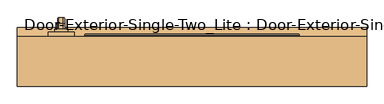
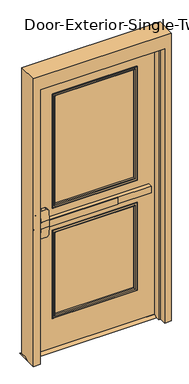
"""IFC4 building model written with IfcOpenShell, lengths in millimetres: door geometry, Door-Exterior-Single-Two_Lite : Door-Exterior-Single-Two_Lite."""

from ifc_helpers import new_model, si_unit, point, frame, frame_2d, origin, place, context, project, spatial, polyline, circle_curve, ellipse_curve, trimmed, segment, composite_curve, outline, extrude, faceted_brep, source, transform, mapped, element, save
from ifc_brep_helpers import plane_surface, cylinder_surface, revolved_surface, advanced_brep


def door_exterior_single_two_lite_door_exterior_single_two_lite_36a17ea7(model_context):
    return source(origin(), model_context, "Body", "SolidModel", [
        extrude(outline(polyline([(38.1, 12.7), (82.55, 12.7), (107.95, 0.0), (12.7, 0.0), (38.1, 12.7)])), frame((-508.0, 0.0, 0.0), z_axis=(1.0, 0.0, 0.0), x_axis=(0.0, 1.0, 0.0)), (0.0, 0.0, 1.0), 1016.0),
        extrude(outline(polyline([(150.2833333, 0.0), (-349.25, 0.0), (-349.25, 6.35), (150.2833333, 6.35), (150.2833333, 0.0)])), frame((0.0, 0.0, 990.6), z_axis=(0.0, 0.0, 1.0), x_axis=(1.0, 0.0, 0.0)), (0.0, 0.0, 1.0), 50.8),
        advanced_brep(
        [(-412.75, 6.35, 1041.4), (-412.75, 6.35, 990.6), (-349.25, 6.35, 990.6), (400.05, 6.35, 990.6), (400.05, 6.35, 1041.4), (-349.25, 6.35, 1041.4), (400.05, 38.1, 1041.4), (400.05, 38.1, 990.6), (-349.25, 38.1, 990.6), (-349.25, 38.1, 927.1), (-368.3, 38.1, 908.05), (-393.7, 38.1, 908.05), (-412.75, 38.1, 927.1), (-412.75, 38.1, 1104.9), (-393.7, 38.1, 1123.95), (-368.3, 38.1, 1123.95), (-349.25, 38.1, 1104.9), (-349.25, 38.1, 1041.4), (-349.25, 9.5252467, 1041.4), (-412.75, 9.5252467, 1041.4), (-412.75, 14.5354269, 1104.9), (-412.75, 14.5354269, 927.1), (-412.75, 9.5252467, 990.6), (-349.25, 9.5252467, 990.6), (-349.25, 14.5354269, 927.1), (-349.25, 14.5354269, 1104.9), (-393.7, 16.038481, 1123.95), (-368.3, 16.038481, 1123.95), (-368.3, 16.038481, 908.05), (-393.7, 16.038481, 908.05)],
        [
            (0, 1),
            (1, 2),
            (2, 3),
            (3, 4),
            (4, 5),
            (5, 0),
            (6, 7),
            (7, 8),
            (8, 9),
            (9, 10, circle_curve(frame((-368.3, 38.1, 927.1), z_axis=(0.0, 1.0, 0.0), x_axis=(1.0, 0.0, 0.0)), 19.05)),
            (10, 11),
            (11, 12, circle_curve(frame((-393.7, 38.1, 927.1), z_axis=(0.0, 1.0, 0.0), x_axis=(1.0, 0.0, 0.0)), 19.05)),
            (12, 13),
            (13, 14, circle_curve(frame((-393.7, 38.1, 1104.9), z_axis=(0.0, 1.0, 0.0), x_axis=(1.0, 0.0, 0.0)), 19.05)),
            (14, 15),
            (15, 16, circle_curve(frame((-368.3, 38.1, 1104.9), z_axis=(0.0, 1.0, 0.0), x_axis=(1.0, 0.0, 0.0)), 19.05)),
            (16, 17),
            (17, 6),
            (4, 6),
            (17, 18),
            (18, 19),
            (19, 0),
            (19, 20),
            (20, 13),
            (12, 21),
            (21, 22),
            (22, 1),
            (7, 3),
            (22, 23),
            (23, 8),
            (23, 24),
            (24, 9),
            (16, 25),
            (25, 18),
            (14, 26),
            (26, 27),
            (27, 15),
            (10, 28),
            (28, 29),
            (29, 11),
            (24, 28, ellipse_curve(frame((-368.3, 14.5354269, 927.1), z_axis=(0.0, 0.9969018152893365, 0.07865602756830282), x_axis=(0.0, -0.07865602756830208, 0.9969018152893365)), 19.1092038, 19.05)),
            (27, 25, ellipse_curve(frame((-368.3, 14.5354269, 1104.9), z_axis=(0.0, 0.9969018152893376, -0.07865602756828934), x_axis=(0.0, -0.078656027568288, -0.9969018152893377)), 19.1092038, 19.05)),
            (20, 26, ellipse_curve(frame((-393.7, 14.5354269, 1104.9), z_axis=(0.0, 0.9969018152893376, -0.07865602756828934), x_axis=(0.0, -0.078656027568288, -0.9969018152893377)), 19.1092038, 19.05)),
            (29, 21, ellipse_curve(frame((-393.7, 14.5354269, 927.1), z_axis=(0.0, 0.9969018152893365, 0.07865602756830282), x_axis=(0.0, -0.07865602756830208, 0.9969018152893365)), 19.1092038, 19.05)),
        ],
        [
            plane_surface(frame((-412.75, 6.35, 1041.4), z_axis=(0.0, -1.0, 0.0), x_axis=(-1.0, 0.0, 0.0))),
            plane_surface(frame((-412.75, 38.1, 1041.4), z_axis=(0.0, 1.0, 0.0), x_axis=(1.0, 0.0, 0.0))),
            plane_surface(frame((400.05, 6.35, 1041.4), z_axis=(0.0, 0.0, 1.0), x_axis=(0.0, 1.0, 0.0))),
            plane_surface(frame((-412.75, 6.35, 1041.4), z_axis=(-1.0, 0.0, 0.0), x_axis=(0.0, 1.0, 0.0))),
            plane_surface(frame((-412.75, 6.35, 990.6), z_axis=(0.0, 0.0, -1.0), x_axis=(0.0, 1.0, 0.0))),
            plane_surface(frame((400.05, 6.35, 990.6), z_axis=(1.0, 0.0, 0.0), x_axis=(0.0, 1.0, 0.0))),
            plane_surface(frame((-349.25, 9.5252467, 927.1), z_axis=(1.0, 0.0, 0.0), x_axis=(0.0, 1.0, 0.0))),
            plane_surface(frame((-368.3, 9.5252467, 1123.95), z_axis=(0.0, 0.0, 1.0), x_axis=(0.0, 1.0, 0.0))),
            plane_surface(frame((-393.7, 9.5252467, 908.05), z_axis=(0.0, 0.0, -1.0), x_axis=(0.0, 1.0, 0.0))),
            cylinder_surface(frame((-368.3, 38.1, 927.1), z_axis=(0.0, -1.0, 0.0), x_axis=(1.0, 0.0, 0.0)), 19.05),
            cylinder_surface(frame((-368.3, 38.1, 1104.9), z_axis=(0.0, -1.0, 0.0), x_axis=(1.0, 0.0, 0.0)), 19.05),
            cylinder_surface(frame((-393.7, 38.1, 1104.9), z_axis=(0.0, -1.0, 0.0), x_axis=(1.0, 0.0, 0.0)), 19.05),
            cylinder_surface(frame((-393.7, 38.1, 927.1), z_axis=(0.0, -1.0, 0.0), x_axis=(1.0, 0.0, 0.0)), 19.05),
            plane_surface(frame((-349.25, 9.5252467, 1041.4), z_axis=(0.0, -0.9969018152893376, 0.07865602756828934), x_axis=(-1.0, 0.0, 0.0))),
            plane_surface(frame((-349.25, 16.038481, 908.05), z_axis=(0.0, -0.9969018152893365, -0.07865602756830282), x_axis=(-1.0, 0.0, 0.0))),
        ],
        [
            (0, [[1, 2, 3, 4, 5, 6]]),
            (1, [[7, 8, 9, 10, 11, 12, 13, 14, 15, 16, 17, 18]]),
            (2, [[19, -18, 20, 21, 22, -6, -5]]),
            (3, [[-1, -22, 23, 24, -13, 25, 26, 27]]),
            (4, [[28, -3, -2, -27, 29, 30, -8]]),
            (5, [[-4, -28, -7, -19]]),
            (6, [[-9, -30, 31, 32]]),
            (6, [[-17, 33, 34, -20]]),
            (7, [[-15, 35, 36, 37]]),
            (8, [[-11, 38, 39, 40]]),
            (9, [[-10, -32, 41, -38]]),
            (10, [[-16, -37, 42, -33]]),
            (11, [[-14, -24, 43, -35]]),
            (12, [[-12, -40, 44, -25]]),
            (13, [[-21, -34, -42, -36, -43, -23]]),
            (14, [[-26, -44, -39, -41, -31, -29]]),
        ],
    ),
        advanced_brep(
        [(-391.0, 95.25, 1017.190625), (-391.0, 95.25, 1014.809375), (-387.428125, 95.25, 1011.2375), (-374.5715406, 95.25, 1011.2375), (-371.0, 95.25, 1014.8090406), (-371.0, 95.25, 1017.190625), (-374.571875, 95.25, 1020.7625), (-387.428125, 95.25, 1020.7625), (-391.0, 95.25, 887.809375), (-387.428125, 95.25, 884.2375), (-374.571875, 95.25, 884.2375), (-371.0, 95.25, 887.809375), (-371.0, 95.25, 890.1909594), (-374.5715406, 95.25, 893.7625), (-387.428125, 95.25, 893.7625), (-391.0, 95.25, 890.190625), (-391.0, 120.65, 1017.190625), (-391.0, 134.540625, 1003.3), (-391.0, 134.540625, 901.7), (-391.0, 120.65, 887.809375), (-391.0, 120.65, 890.190625), (-391.0, 132.159375, 901.7), (-391.0, 132.159375, 1003.3), (-391.0, 120.65, 1014.809375), (-387.428125, 120.65, 1011.2375), (-374.5715406, 120.65, 1011.2375), (-371.0, 120.65, 1014.8090406), (-371.0, 132.1590406, 1003.3), (-371.0, 132.1590406, 901.7), (-371.0, 120.65, 890.1909594), (-371.0, 120.65, 887.809375), (-371.0, 134.540625, 901.7), (-371.0, 134.540625, 1003.3), (-371.0, 120.65, 1017.190625), (-374.571875, 120.65, 1020.7625), (-387.428125, 120.65, 1020.7625), (-387.428125, 128.5875, 1003.3), (-374.5715406, 128.5875, 1003.3), (-374.571875, 138.1125, 1003.3), (-387.428125, 138.1125, 1003.3), (-387.428125, 128.5875, 901.7), (-374.5715406, 128.5875, 901.7), (-374.571875, 138.1125, 901.7), (-387.428125, 138.1125, 901.7), (-387.428125, 120.65, 893.7625), (-374.5715406, 120.65, 893.7625), (-374.571875, 120.65, 884.2375), (-387.428125, 120.65, 884.2375)],
        [
            (0, 1),
            (1, 2, circle_curve(frame((-387.428125, 95.25, 1014.809375), z_axis=(0.0, -1.0, 0.0), x_axis=(0.0, 0.0, 1.0)), 3.571875)),
            (2, 3),
            (3, 4, circle_curve(frame((-374.5715406, 95.25, 1014.8090406), z_axis=(0.0, -1.0, 0.0), x_axis=(0.0, 0.0, 1.0)), 3.5715406)),
            (4, 5),
            (5, 6, circle_curve(frame((-374.571875, 95.25, 1017.190625), z_axis=(0.0, -1.0, 0.0), x_axis=(0.0, 0.0, 1.0)), 3.571875)),
            (6, 7),
            (7, 0, circle_curve(frame((-387.428125, 95.25, 1017.190625), z_axis=(0.0, -1.0, 0.0), x_axis=(0.0, 0.0, 1.0)), 3.571875)),
            (8, 9, circle_curve(frame((-387.428125, 95.25, 887.809375), z_axis=(0.0, -1.0, 0.0), x_axis=(0.0, 0.0, -1.0)), 3.571875)),
            (9, 10),
            (10, 11, circle_curve(frame((-374.571875, 95.25, 887.809375), z_axis=(0.0, -1.0, 0.0), x_axis=(0.0, 0.0, -1.0)), 3.571875)),
            (11, 12),
            (12, 13, circle_curve(frame((-374.5715406, 95.25, 890.1909594), z_axis=(0.0, -1.0, 0.0), x_axis=(0.0, 0.0, -1.0)), 3.5715406)),
            (13, 14),
            (14, 15, circle_curve(frame((-387.428125, 95.25, 890.190625), z_axis=(0.0, -1.0, 0.0), x_axis=(0.0, 0.0, -1.0)), 3.571875)),
            (15, 8),
            (0, 16),
            (16, 17, circle_curve(frame((-391.0, 120.65, 1003.3), z_axis=(-1.0, 0.0, 0.0), x_axis=(0.0, 0.0, 1.0)), 13.890625)),
            (17, 18),
            (18, 19, circle_curve(frame((-391.0, 120.65, 901.7), z_axis=(-1.0, 0.0, 0.0), x_axis=(0.0, 1.0, 0.0)), 13.890625)),
            (19, 8),
            (15, 20),
            (20, 21, circle_curve(frame((-391.0, 120.65, 901.7), z_axis=(1.0, 0.0, 0.0), x_axis=(0.0, 1.0, 0.0)), 11.509375)),
            (21, 22),
            (22, 23, circle_curve(frame((-391.0, 120.65, 1003.3), z_axis=(1.0, 0.0, 0.0), x_axis=(0.0, 0.0, 1.0)), 11.509375)),
            (23, 1),
            (23, 24, circle_curve(frame((-387.428125, 120.65, 1014.809375), z_axis=(0.0, -1.0, 0.0), x_axis=(0.0, 0.0, 1.0)), 3.571875)),
            (24, 2),
            (24, 25),
            (25, 3),
            (25, 26, circle_curve(frame((-374.5715406, 120.65, 1014.8090406), z_axis=(0.0, -1.0, 0.0), x_axis=(0.0, 0.0, 1.0)), 3.5715406)),
            (26, 4),
            (26, 27, circle_curve(frame((-371.0, 120.65, 1003.3), z_axis=(-1.0, 0.0, 0.0), x_axis=(0.0, 0.0, 1.0)), 11.5090406)),
            (27, 28),
            (28, 29, circle_curve(frame((-371.0, 120.65, 901.7), z_axis=(-1.0, 0.0, 0.0), x_axis=(0.0, 1.0, 0.0)), 11.5090406)),
            (29, 12),
            (11, 30),
            (30, 31, circle_curve(frame((-371.0, 120.65, 901.7), z_axis=(1.0, 0.0, 0.0), x_axis=(0.0, 1.0, 0.0)), 13.890625)),
            (31, 32),
            (32, 33, circle_curve(frame((-371.0, 120.65, 1003.3), z_axis=(1.0, 0.0, 0.0), x_axis=(0.0, 0.0, 1.0)), 13.890625)),
            (33, 5),
            (33, 34, circle_curve(frame((-374.571875, 120.65, 1017.190625), z_axis=(0.0, -1.0, 0.0), x_axis=(0.0, 0.0, 1.0)), 3.571875)),
            (34, 6),
            (34, 35),
            (35, 7),
            (35, 16, circle_curve(frame((-387.428125, 120.65, 1017.190625), z_axis=(0.0, -1.0, 0.0), x_axis=(0.0, 0.0, 1.0)), 3.571875)),
            (36, 24, circle_curve(frame((-387.428125, 120.65, 1003.3), z_axis=(1.0, 0.0, 0.0), x_axis=(0.0, 0.0, 1.0)), 7.9375)),
            (22, 36, circle_curve(frame((-387.428125, 132.159375, 1003.3), z_axis=(0.0, 0.0, 1.0), x_axis=(0.0, 1.0, 0.0)), 3.571875)),
            (37, 25, circle_curve(frame((-374.5715406, 120.65, 1003.3), z_axis=(1.0, 0.0, 0.0), x_axis=(0.0, 0.0, 1.0)), 7.9375)),
            (36, 37),
            (37, 27, circle_curve(frame((-374.5715406, 132.1590406, 1003.3), z_axis=(0.0, 0.0, 1.0), x_axis=(0.0, 1.0, 0.0)), 3.5715406)),
            (38, 34, circle_curve(frame((-374.571875, 120.65, 1003.3), z_axis=(1.0, 0.0, 0.0), x_axis=(0.0, 0.0, 1.0)), 17.4625)),
            (32, 38, circle_curve(frame((-374.571875, 134.540625, 1003.3), z_axis=(0.0, 0.0, 1.0), x_axis=(0.0, 1.0, 0.0)), 3.571875)),
            (39, 35, circle_curve(frame((-387.428125, 120.65, 1003.3), z_axis=(1.0, 0.0, 0.0), x_axis=(0.0, 0.0, 1.0)), 17.4625)),
            (38, 39),
            (39, 17, circle_curve(frame((-387.428125, 134.540625, 1003.3), z_axis=(0.0, 0.0, 1.0), x_axis=(0.0, 1.0, 0.0)), 3.571875)),
            (21, 40, circle_curve(frame((-387.428125, 132.159375, 901.7), z_axis=(0.0, 0.0, 1.0), x_axis=(0.0, 1.0, 0.0)), 3.571875)),
            (40, 36),
            (40, 41),
            (41, 37),
            (41, 28, circle_curve(frame((-374.5715406, 132.1590406, 901.7), z_axis=(0.0, 0.0, 1.0), x_axis=(0.0, 1.0, 0.0)), 3.5715406)),
            (31, 42, circle_curve(frame((-374.571875, 134.540625, 901.7), z_axis=(0.0, 0.0, 1.0), x_axis=(0.0, 1.0, 0.0)), 3.571875)),
            (42, 38),
            (42, 43),
            (43, 39),
            (43, 18, circle_curve(frame((-387.428125, 134.540625, 901.7), z_axis=(0.0, 0.0, 1.0), x_axis=(0.0, 1.0, 0.0)), 3.571875)),
            (44, 40, circle_curve(frame((-387.428125, 120.65, 901.7), z_axis=(1.0, 0.0, 0.0), x_axis=(0.0, 1.0, 0.0)), 7.9375)),
            (20, 44, circle_curve(frame((-387.428125, 120.65, 890.190625), z_axis=(0.0, 1.0, 0.0), x_axis=(0.0, 0.0, -1.0)), 3.571875)),
            (45, 41, circle_curve(frame((-374.5715406, 120.65, 901.7), z_axis=(1.0, 0.0, 0.0), x_axis=(0.0, 1.0, 0.0)), 7.9375)),
            (44, 45),
            (45, 29, circle_curve(frame((-374.5715406, 120.65, 890.1909594), z_axis=(0.0, 1.0, 0.0), x_axis=(0.0, 0.0, -1.0)), 3.5715406)),
            (46, 42, circle_curve(frame((-374.571875, 120.65, 901.7), z_axis=(1.0, 0.0, 0.0), x_axis=(0.0, 1.0, 0.0)), 17.4625)),
            (30, 46, circle_curve(frame((-374.571875, 120.65, 887.809375), z_axis=(0.0, 1.0, 0.0), x_axis=(0.0, 0.0, -1.0)), 3.571875)),
            (47, 43, circle_curve(frame((-387.428125, 120.65, 901.7), z_axis=(1.0, 0.0, 0.0), x_axis=(0.0, 1.0, 0.0)), 17.4625)),
            (46, 47),
            (47, 19, circle_curve(frame((-387.428125, 120.65, 887.809375), z_axis=(0.0, 1.0, 0.0), x_axis=(0.0, 0.0, -1.0)), 3.571875)),
            (14, 44),
            (13, 45),
            (10, 46),
            (9, 47),
        ],
        [
            plane_surface(frame((-381.0, 95.25, 1016.0), z_axis=(0.0, -1.0, 0.0), x_axis=(1.0, 0.0, 0.0))),
            plane_surface(frame((-381.0, 95.25, 889.0), z_axis=(0.0, -1.0, 0.0), x_axis=(1.0, 0.0, 0.0))),
            plane_surface(frame((-391.0, 95.25, 1017.190625), z_axis=(-1.0, 0.0, 0.0), x_axis=(0.0, 1.0, 0.0))),
            cylinder_surface(frame((-387.428125, 95.25, 1014.809375), z_axis=(0.0, -1.0, 0.0), x_axis=(0.0, 0.0, 1.0)), 3.571875),
            plane_surface(frame((-387.428125, 95.25, 1011.2375), z_axis=(0.0, 0.0, -1.0), x_axis=(0.0, 1.0, 0.0))),
            cylinder_surface(frame((-374.5715406, 95.25, 1014.8090406), z_axis=(0.0, -1.0, 0.0), x_axis=(0.0, 0.0, 1.0)), 3.5715406),
            plane_surface(frame((-371.0, 95.25, 1014.8090406), z_axis=(1.0, 0.0, 0.0), x_axis=(0.0, 1.0, 0.0))),
            cylinder_surface(frame((-374.571875, 95.25, 1017.190625), z_axis=(0.0, -1.0, 0.0), x_axis=(0.0, 0.0, 1.0)), 3.571875),
            plane_surface(frame((-374.571875, 95.25, 1020.7625), z_axis=(0.0, 0.0, 1.0), x_axis=(0.0, 1.0, 0.0))),
            cylinder_surface(frame((-387.428125, 95.25, 1017.190625), z_axis=(0.0, -1.0, 0.0), x_axis=(0.0, 0.0, 1.0)), 3.571875),
            revolved_surface(trimmed(ellipse_curve(frame((-387.428125, 120.65, 1014.809375), z_axis=(0.0, -1.0, 0.0), x_axis=(0.0, 0.0, 1.0)), 3.571875, 3.571875), [point((-391.0, 120.65, 1014.809375))], [point((-387.428125, 120.65, 1011.2375))], True, "CARTESIAN"), (-381.0, 120.65, 1003.3), (-1.0, 0.0, 0.0)),
            revolved_surface(polyline([(-387.428125, 120.65, 1011.2375), (-374.5715406, 120.65, 1011.2375)]), (-381.0, 120.65, 1003.3), (-1.0, 0.0, 0.0)),
            revolved_surface(trimmed(ellipse_curve(frame((-374.5715406, 120.65, 1014.8090406), z_axis=(0.0, -1.0, 0.0), x_axis=(0.0, 0.0, 1.0)), 3.5715406, 3.5715406), [point((-374.5715406, 120.65, 1011.2375))], [point((-371.0, 120.65, 1014.8090406))], True, "CARTESIAN"), (-381.0, 120.65, 1003.3), (-1.0, 0.0, 0.0)),
            revolved_surface(trimmed(ellipse_curve(frame((-374.571875, 120.65, 1017.190625), z_axis=(0.0, -1.0, 0.0), x_axis=(0.0, 0.0, 1.0)), 3.571875, 3.571875), [point((-371.0, 120.65, 1017.190625))], [point((-374.571875, 120.65, 1020.7625))], True, "CARTESIAN"), (-381.0, 120.65, 1003.3), (-1.0, 0.0, 0.0)),
            cylinder_surface(frame((-381.0, 120.65, 1003.3), z_axis=(-1.0, 0.0, 0.0), x_axis=(0.0, 0.0, 1.0)), 17.4625),
            revolved_surface(trimmed(ellipse_curve(frame((-387.428125, 120.65, 1017.190625), z_axis=(0.0, -1.0, 0.0), x_axis=(0.0, 0.0, 1.0)), 3.571875, 3.571875), [point((-387.428125, 120.65, 1020.7625))], [point((-391.0, 120.65, 1017.190625))], True, "CARTESIAN"), (-381.0, 120.65, 1003.3), (-1.0, 0.0, 0.0)),
            cylinder_surface(frame((-387.428125, 132.159375, 1003.3), z_axis=(0.0, 0.0, 1.0), x_axis=(0.0, 1.0, 0.0)), 3.571875),
            plane_surface(frame((-387.428125, 128.5875, 1003.3), z_axis=(0.0, -1.0, 0.0), x_axis=(0.0, 0.0, -1.0))),
            cylinder_surface(frame((-374.5715406, 132.1590406, 1003.3), z_axis=(0.0, 0.0, 1.0), x_axis=(0.0, 1.0, 0.0)), 3.5715406),
            cylinder_surface(frame((-374.571875, 134.540625, 1003.3), z_axis=(0.0, 0.0, 1.0), x_axis=(0.0, 1.0, 0.0)), 3.571875),
            plane_surface(frame((-374.571875, 138.1125, 1003.3), z_axis=(0.0, 1.0, 0.0), x_axis=(0.0, 0.0, -1.0))),
            cylinder_surface(frame((-387.428125, 134.540625, 1003.3), z_axis=(0.0, 0.0, 1.0), x_axis=(0.0, 1.0, 0.0)), 3.571875),
            revolved_surface(trimmed(ellipse_curve(frame((-387.428125, 132.159375, 901.7), z_axis=(0.0, 0.0, 1.0), x_axis=(0.0, 1.0, 0.0)), 3.571875, 3.571875), [point((-391.0, 132.159375, 901.7))], [point((-387.428125, 128.5875, 901.7))], True, "CARTESIAN"), (-381.0, 120.65, 901.7), (-1.0, 0.0, 0.0)),
            revolved_surface(polyline([(-387.428125, 128.5875, 901.7), (-374.5715406, 128.5875, 901.7)]), (-381.0, 120.65, 901.7), (-1.0, 0.0, 0.0)),
            revolved_surface(trimmed(ellipse_curve(frame((-374.5715406, 132.1590406, 901.7), z_axis=(0.0, 0.0, 1.0), x_axis=(0.0, 1.0, 0.0)), 3.5715406, 3.5715406), [point((-374.5715406, 128.5875, 901.7))], [point((-371.0, 132.1590406, 901.7))], True, "CARTESIAN"), (-381.0, 120.65, 901.7), (-1.0, 0.0, 0.0)),
            revolved_surface(trimmed(ellipse_curve(frame((-374.571875, 134.540625, 901.7), z_axis=(0.0, 0.0, 1.0), x_axis=(0.0, 1.0, 0.0)), 3.571875, 3.571875), [point((-371.0, 134.540625, 901.7))], [point((-374.571875, 138.1125, 901.7))], True, "CARTESIAN"), (-381.0, 120.65, 901.7), (-1.0, 0.0, 0.0)),
            cylinder_surface(frame((-381.0, 120.65, 901.7), z_axis=(-1.0, 0.0, 0.0), x_axis=(0.0, 1.0, 0.0)), 17.4625),
            revolved_surface(trimmed(ellipse_curve(frame((-387.428125, 134.540625, 901.7), z_axis=(0.0, 0.0, 1.0), x_axis=(0.0, 1.0, 0.0)), 3.571875, 3.571875), [point((-387.428125, 138.1125, 901.7))], [point((-391.0, 134.540625, 901.7))], True, "CARTESIAN"), (-381.0, 120.65, 901.7), (-1.0, 0.0, 0.0)),
            cylinder_surface(frame((-387.428125, 120.65, 890.190625), z_axis=(0.0, 1.0, 0.0), x_axis=(0.0, 0.0, -1.0)), 3.571875),
            plane_surface(frame((-387.428125, 120.65, 893.7625), z_axis=(0.0, 0.0, 1.0), x_axis=(0.0, -1.0, 0.0))),
            cylinder_surface(frame((-374.5715406, 120.65, 890.1909594), z_axis=(0.0, 1.0, 0.0), x_axis=(0.0, 0.0, -1.0)), 3.5715406),
            cylinder_surface(frame((-374.571875, 120.65, 887.809375), z_axis=(0.0, 1.0, 0.0), x_axis=(0.0, 0.0, -1.0)), 3.571875),
            plane_surface(frame((-374.571875, 120.65, 884.2375), z_axis=(0.0, 0.0, -1.0), x_axis=(0.0, -1.0, 0.0))),
            cylinder_surface(frame((-387.428125, 120.65, 887.809375), z_axis=(0.0, 1.0, 0.0), x_axis=(0.0, 0.0, -1.0)), 3.571875),
        ],
        [
            (0, [[1, 2, 3, 4, 5, 6, 7, 8]]),
            (1, [[9, 10, 11, 12, 13, 14, 15, 16]]),
            (2, [[-1, 17, 18, 19, 20, 21, -16, 22, 23, 24, 25, 26]]),
            (3, [[-2, -26, 27, 28]]),
            (4, [[-3, -28, 29, 30]]),
            (5, [[-4, -30, 31, 32]]),
            (6, [[-5, -32, 33, 34, 35, 36, -12, 37, 38, 39, 40, 41]]),
            (7, [[-6, -41, 42, 43]]),
            (8, [[-7, -43, 44, 45]]),
            (9, [[-8, -45, 46, -17]]),
            (10, [[47, -27, -25, 48]]),
            (11, [[49, -29, -47, 50]]),
            (12, [[-33, -31, -49, 51]]),
            (13, [[52, -42, -40, 53]]),
            (14, [[54, -44, -52, 55]]),
            (15, [[-18, -46, -54, 56]]),
            (16, [[-48, -24, 57, 58]]),
            (17, [[-50, -58, 59, 60]]),
            (18, [[-51, -60, 61, -34]]),
            (19, [[-53, -39, 62, 63]]),
            (20, [[-55, -63, 64, 65]]),
            (21, [[-56, -65, 66, -19]]),
            (22, [[67, -57, -23, 68]]),
            (23, [[69, -59, -67, 70]]),
            (24, [[-35, -61, -69, 71]]),
            (25, [[72, -62, -38, 73]]),
            (26, [[74, -64, -72, 75]]),
            (27, [[-20, -66, -74, 76]]),
            (28, [[-68, -22, -15, 77]]),
            (29, [[-70, -77, -14, 78]]),
            (30, [[-71, -78, -13, -36]]),
            (31, [[-73, -37, -11, 79]]),
            (32, [[-75, -79, -10, 80]]),
            (33, [[-76, -80, -9, -21]]),
        ],
    ),
        extrude(outline(composite_curve([segment(trimmed(circle_curve(frame_2d((1117.6, -381.0)), 19.0), [point((1117.6, -400.0))], [point((1117.6, -362.0))], False, "CARTESIAN"), True, "CONTINUOUS"), segment(trimmed(circle_curve(frame_2d((1117.6, -381.0)), 19.0), [point((1117.6, -362.0))], [point((1117.6, -400.0))], False, "CARTESIAN"), True, "CONTINUOUS")], self_intersect=False)), frame((0.0, 95.25, 0.0), z_axis=(0.0, 1.0, 0.0), x_axis=(0.0, 0.0, 1.0)), (0.0, 0.0, 1.0), 8.73125),
        extrude(outline(composite_curve([segment(trimmed(circle_curve(frame_2d((1113.0338574, -381.0)), 89.3016225), [point((1193.8, -342.9))], [point((1193.8, -419.1))], False, "CARTESIAN"), True, "CONTINUOUS"), segment(polyline([(1193.8, -419.1), (838.2, -419.1)]), True, "CONTINUOUS"), segment(trimmed(circle_curve(frame_2d((918.9661426, -381.0)), 89.3016225), [point((838.2, -419.1))], [point((838.2, -342.9))], False, "CARTESIAN"), True, "CONTINUOUS"), segment(polyline([(838.2, -342.9), (1193.8, -342.9)]), True, "CONTINUOUS")], self_intersect=False)), frame((0.0, 82.55, 0.0), z_axis=(0.0, 1.0, 0.0), x_axis=(0.0, 0.0, 1.0)), (0.0, 0.0, 1.0), 12.7),
        faceted_brep([(457.2, 33.3375, 0.0), (457.2, 82.55, 0.0), (508.0, 82.55, 0.0), (508.0, -63.5, 0.0), (457.2, -63.5, 0.0), (457.2, -14.2875, 0.0), (441.325, -14.2875, 0.0), (441.325, 33.3375, 0.0), (457.2, 33.3375, 2133.6), (457.2, 82.55, 2133.6), (-457.2, 82.55, 2133.6), (-457.2, 82.55, 0.0), (-508.0, 82.55, 0.0), (-508.0, 82.55, 2235.2), (508.0, 82.55, 2235.2), (508.0, -63.5, 2235.2), (-508.0, -63.5, 2235.2), (-508.0, -63.5, 0.0), (-457.2, -63.5, 0.0), (-457.2, -63.5, 2133.6), (457.2, -63.5, 2133.6), (457.2, -14.2875, 2133.6), (-457.2, -14.2875, 2133.6), (-457.2, -14.2875, 0.0), (-441.325, -14.2875, 0.0), (-441.325, -14.2875, 2117.725), (441.325, -14.2875, 2117.725), (441.325, 33.3375, 2117.725), (-441.325, 33.3375, 2117.725), (-441.325, 33.3375, 0.0), (-457.2, 33.3375, 0.0), (-457.2, 33.3375, 2133.6)], [[[0, 1, 2, 3, 4, 5, 6, 7]], [[1, 0, 8, 9]], [[2, 1, 9, 10, 11, 12, 13, 14]], [[3, 2, 14, 15]], [[4, 3, 15, 16, 17, 18, 19, 20]], [[5, 4, 20, 21]], [[6, 5, 21, 22, 23, 24, 25, 26]], [[7, 6, 26, 27]], [[0, 7, 27, 28, 29, 30, 31, 8]], [[9, 8, 31, 10]], [[20, 19, 22, 21]], [[26, 25, 28, 27]], [[12, 11, 30, 29, 24, 23, 18, 17]], [[11, 10, 31, 30]], [[13, 12, 17, 16]], [[19, 18, 23, 22]], [[25, 24, 29, 28]], [[15, 14, 13, 16]]]),
        extrude(outline(polyline([(2133.6, -457.2), (12.7, -457.2), (12.7, 457.2), (2133.6, 457.2), (2133.6, -457.2)]), holes=[polyline([(1981.2, -304.8), (1981.2, 304.8), (1111.25, 304.8), (1111.25, -304.8), (1981.2, -304.8)]), polyline([(920.75, -304.8), (920.75, 304.8), (254.0, 304.8), (254.0, -304.8), (920.75, -304.8)])]), frame((0.0, 38.1, 0.0), z_axis=(0.0, 1.0, 0.0), x_axis=(0.0, 0.0, 1.0)), (0.0, 0.0, 1.0), 44.45),
        extrude(outline(polyline([(304.8, 50.8), (-304.8, 50.8), (-304.8, 69.85), (304.8, 69.85), (304.8, 50.8)])), frame((0.0, 0.0, 1111.25), z_axis=(0.0, 0.0, 1.0), x_axis=(1.0, 0.0, 0.0)), (0.0, 0.0, 1.0), 869.95),
        extrude(outline(polyline([(304.8, 50.8), (-304.8, 50.8), (-304.8, 69.85), (304.8, 69.85), (304.8, 50.8)])), frame((0.0, 0.0, 254.0), z_axis=(0.0, 0.0, 1.0), x_axis=(1.0, 0.0, 0.0)), (0.0, 0.0, 1.0), 666.75),
        advanced_brep(
        [(304.8, 50.8, 920.75), (304.8, 38.1, 920.75), (304.8, 38.1, 254.0), (304.8, 50.8, 254.0), (292.8, 37.1, 908.75), (292.8, 50.8, 908.75), (292.8, 50.8, 266.0), (292.8, 37.1, 266.0), (297.8, 32.1, 913.75), (297.8, 32.1, 261.0), (312.8, 34.1, 928.75), (310.8, 32.1, 926.75), (310.8, 32.1, 248.0), (312.8, 34.1, 246.0), (312.8, 38.1, 928.75), (312.8, 38.1, 246.0), (-304.8, 38.1, 254.0), (-304.8, 50.8, 254.0), (-292.8, 50.8, 266.0), (-292.8, 37.1, 266.0), (-297.8, 32.1, 261.0), (-310.8, 32.1, 248.0), (-312.8, 34.1, 246.0), (-312.8, 38.1, 246.0), (-304.8, 38.1, 920.75), (-304.8, 50.8, 920.75), (-292.8, 50.8, 908.75), (-292.8, 37.1, 908.75), (-297.8, 32.1, 913.75), (-310.8, 32.1, 926.75), (-312.8, 34.1, 928.75), (-312.8, 38.1, 928.75)],
        [
            (0, 1),
            (1, 2),
            (2, 3),
            (3, 0),
            (4, 5),
            (5, 6),
            (6, 7),
            (7, 4),
            (8, 4, ellipse_curve(frame((297.8, 37.1, 913.75), z_axis=(0.7071067811865475, 0.0, -0.7071067811865475), x_axis=(0.7071067811865474, 0.0, 0.7071067811865476)), 7.0710678, 5.0)),
            (7, 9, ellipse_curve(frame((297.8, 37.1, 261.0), z_axis=(0.7071067811865475, 0.0, 0.7071067811865475), x_axis=(-0.7071067811865474, 0.0, 0.7071067811865476)), 7.0710678, 5.0)),
            (9, 8),
            (10, 11, ellipse_curve(frame((310.8, 34.1, 926.75), z_axis=(0.7071067811865475, 0.0, -0.7071067811865475), x_axis=(0.7071067811865474, 0.0, 0.7071067811865476)), 2.8284271, 2.0)),
            (11, 12),
            (12, 13, ellipse_curve(frame((310.8, 34.1, 248.0), z_axis=(0.7071067811865475, 0.0, 0.7071067811865475), x_axis=(-0.7071067811865474, 0.0, 0.7071067811865476)), 2.8284271, 2.0)),
            (13, 10),
            (14, 10),
            (13, 15),
            (15, 14),
            (2, 16),
            (16, 17),
            (17, 3),
            (6, 18),
            (18, 19),
            (19, 7),
            (19, 20, ellipse_curve(frame((-297.8, 37.1, 261.0), z_axis=(0.7071067811865475, 0.0, -0.7071067811865475), x_axis=(0.7071067811865476, 0.0, 0.7071067811865474)), 7.0710678, 5.0)),
            (20, 9),
            (12, 21),
            (21, 22, ellipse_curve(frame((-310.8, 34.1, 248.0), z_axis=(0.7071067811865475, 0.0, -0.7071067811865475), x_axis=(0.7071067811865476, 0.0, 0.7071067811865474)), 2.8284271, 2.0)),
            (22, 13),
            (22, 23),
            (23, 15),
            (16, 24),
            (24, 25),
            (25, 17),
            (18, 26),
            (26, 27),
            (27, 19),
            (27, 28, ellipse_curve(frame((-297.8, 37.1, 913.75), z_axis=(-0.7071067811865475, 0.0, -0.7071067811865475), x_axis=(0.7071067811865474, 0.0, -0.7071067811865476)), 7.0710678, 5.0)),
            (28, 20),
            (21, 29),
            (29, 30, ellipse_curve(frame((-310.8, 34.1, 926.75), z_axis=(-0.7071067811865475, 0.0, -0.7071067811865475), x_axis=(0.7071067811865474, 0.0, -0.7071067811865476)), 2.8284271, 2.0)),
            (30, 22),
            (30, 31),
            (31, 23),
            (31, 14),
            (1, 24),
            (0, 25),
            (5, 26),
            (4, 27),
            (8, 28),
            (11, 29),
            (10, 30),
        ],
        [
            plane_surface(frame((304.8, 38.1, 920.75), z_axis=(1.0, 0.0, 0.0), x_axis=(0.0, 0.0, -1.0))),
            plane_surface(frame((292.8, 50.8, 908.75), z_axis=(-1.0, 0.0, 0.0), x_axis=(0.0, 0.0, -1.0))),
            cylinder_surface(frame((297.8, 37.1, 920.75), z_axis=(0.0, 0.0, 1.0), x_axis=(1.0, 0.0, 0.0)), 5.0),
            cylinder_surface(frame((310.8, 34.1, 920.75), z_axis=(0.0, 0.0, 1.0), x_axis=(1.0, 0.0, 0.0)), 2.0),
            plane_surface(frame((312.8, 34.1, 928.75), z_axis=(1.0, 0.0, 0.0), x_axis=(0.0, 0.0, -1.0))),
            plane_surface(frame((304.8, 38.1, 254.0), z_axis=(0.0, 0.0, -1.0), x_axis=(-1.0, 0.0, 0.0))),
            plane_surface(frame((292.8, 50.8, 266.0), z_axis=(0.0, 0.0, 1.0), x_axis=(-1.0, 0.0, 0.0))),
            cylinder_surface(frame((304.8, 37.1, 261.0), z_axis=(1.0, 0.0, 0.0), x_axis=(0.0, 0.0, -1.0)), 5.0),
            cylinder_surface(frame((304.8, 34.1, 248.0), z_axis=(1.0, 0.0, 0.0), x_axis=(0.0, 0.0, -1.0)), 2.0),
            plane_surface(frame((312.8, 34.1, 246.0), z_axis=(0.0, 0.0, -1.0), x_axis=(-1.0, 0.0, 0.0))),
            plane_surface(frame((-304.8, 38.1, 254.0), z_axis=(-1.0, 0.0, 0.0), x_axis=(0.0, 0.0, 1.0))),
            plane_surface(frame((-292.8, 50.8, 266.0), z_axis=(1.0, 0.0, 0.0), x_axis=(0.0, 0.0, 1.0))),
            cylinder_surface(frame((-297.8, 37.1, 254.0), z_axis=(0.0, 0.0, -1.0), x_axis=(-1.0, 0.0, 0.0)), 5.0),
            cylinder_surface(frame((-310.8, 34.1, 254.0), z_axis=(0.0, 0.0, -1.0), x_axis=(-1.0, 0.0, 0.0)), 2.0),
            plane_surface(frame((-312.8, 34.1, 246.0), z_axis=(-1.0, 0.0, 0.0), x_axis=(0.0, 0.0, 1.0))),
            plane_surface(frame((-312.8, 38.1, 928.75), z_axis=(0.0, 1.0, 0.0), x_axis=(1.0, 0.0, 0.0))),
            plane_surface(frame((-304.8, 38.1, 920.75), z_axis=(0.0, 0.0, 1.0), x_axis=(1.0, 0.0, 0.0))),
            plane_surface(frame((-304.8, 50.8, 920.75), z_axis=(0.0, 1.0, 0.0), x_axis=(1.0, 0.0, 0.0))),
            plane_surface(frame((-292.8, 50.8, 908.75), z_axis=(0.0, 0.0, -1.0), x_axis=(1.0, 0.0, 0.0))),
            cylinder_surface(frame((-304.8, 37.1, 913.75), z_axis=(-1.0, 0.0, 0.0), x_axis=(0.0, 0.0, 1.0)), 5.0),
            plane_surface(frame((-297.8, 32.1, 913.75), z_axis=(0.0, -1.0, 0.0), x_axis=(1.0, 0.0, 0.0))),
            cylinder_surface(frame((-304.8, 34.1, 926.75), z_axis=(-1.0, 0.0, 0.0), x_axis=(0.0, 0.0, 1.0)), 2.0),
            plane_surface(frame((-312.8, 34.1, 928.75), z_axis=(0.0, 0.0, 1.0), x_axis=(1.0, 0.0, 0.0))),
        ],
        [
            (0, [[1, 2, 3, 4]]),
            (1, [[5, 6, 7, 8]]),
            (2, [[9, -8, 10, 11]]),
            (3, [[12, 13, 14, 15]]),
            (4, [[16, -15, 17, 18]]),
            (5, [[-3, 19, 20, 21]]),
            (6, [[-7, 22, 23, 24]]),
            (7, [[-10, -24, 25, 26]]),
            (8, [[-14, 27, 28, 29]]),
            (9, [[-17, -29, 30, 31]]),
            (10, [[-20, 32, 33, 34]]),
            (11, [[-23, 35, 36, 37]]),
            (12, [[-25, -37, 38, 39]]),
            (13, [[-28, 40, 41, 42]]),
            (14, [[-30, -42, 43, 44]]),
            (15, [[-31, -44, 45, -18], [46, -32, -19, -2]]),
            (16, [[-33, -46, -1, 47]]),
            (17, [[-21, -34, -47, -4], [48, -35, -22, -6]]),
            (18, [[-36, -48, -5, 49]]),
            (19, [[-38, -49, -9, 50]]),
            (20, [[51, -40, -27, -13], [-26, -39, -50, -11]]),
            (21, [[-41, -51, -12, 52]]),
            (22, [[-43, -52, -16, -45]]),
        ],
    ),
        advanced_brep(
        [(-304.8, 69.85, 920.75), (-304.8, 82.55, 920.75), (-304.8, 82.55, 254.0), (-304.8, 69.85, 254.0), (-292.8, 83.55, 908.75), (-292.8, 69.85, 908.75), (-292.8, 69.85, 266.0), (-292.8, 83.55, 266.0), (-297.8, 88.55, 913.75), (-297.8, 88.55, 261.0), (-312.8, 86.55, 928.75), (-310.8, 88.55, 926.75), (-310.8, 88.55, 248.0), (-312.8, 86.55, 246.0), (-312.8, 82.55, 928.75), (-312.8, 82.55, 246.0), (304.8, 82.55, 254.0), (304.8, 69.85, 254.0), (292.8, 69.85, 266.0), (292.8, 83.55, 266.0), (297.8, 88.55, 261.0), (310.8, 88.55, 248.0), (312.8, 86.55, 246.0), (312.8, 82.55, 246.0), (304.8, 82.55, 920.75), (304.8, 69.85, 920.75), (292.8, 69.85, 908.75), (292.8, 83.55, 908.75), (297.8, 88.55, 913.75), (310.8, 88.55, 926.75), (312.8, 86.55, 928.75), (312.8, 82.55, 928.75)],
        [
            (0, 1),
            (1, 2),
            (2, 3),
            (3, 0),
            (4, 5),
            (5, 6),
            (6, 7),
            (7, 4),
            (8, 4, ellipse_curve(frame((-297.8, 83.55, 913.75), z_axis=(-0.7071067811865475, 0.0, -0.7071067811865475), x_axis=(-0.7071067811865474, 0.0, 0.7071067811865476)), 7.0710678, 5.0)),
            (7, 9, ellipse_curve(frame((-297.8, 83.55, 261.0), z_axis=(-0.7071067811865475, 0.0, 0.7071067811865475), x_axis=(0.7071067811865474, 0.0, 0.7071067811865476)), 7.0710678, 5.0)),
            (9, 8),
            (10, 11, ellipse_curve(frame((-310.8, 86.55, 926.75), z_axis=(-0.7071067811865475, 0.0, -0.7071067811865475), x_axis=(-0.7071067811865474, 0.0, 0.7071067811865476)), 2.8284271, 2.0)),
            (11, 12),
            (12, 13, ellipse_curve(frame((-310.8, 86.55, 248.0), z_axis=(-0.7071067811865475, 0.0, 0.7071067811865475), x_axis=(0.7071067811865474, 0.0, 0.7071067811865476)), 2.8284271, 2.0)),
            (13, 10),
            (14, 10),
            (13, 15),
            (15, 14),
            (2, 16),
            (16, 17),
            (17, 3),
            (6, 18),
            (18, 19),
            (19, 7),
            (19, 20, ellipse_curve(frame((297.8, 83.55, 261.0), z_axis=(-0.7071067811865475, 0.0, -0.7071067811865475), x_axis=(-0.7071067811865476, 0.0, 0.7071067811865474)), 7.0710678, 5.0)),
            (20, 9),
            (12, 21),
            (21, 22, ellipse_curve(frame((310.8, 86.55, 248.0), z_axis=(-0.7071067811865475, 0.0, -0.7071067811865475), x_axis=(-0.7071067811865476, 0.0, 0.7071067811865474)), 2.8284271, 2.0)),
            (22, 13),
            (22, 23),
            (23, 15),
            (16, 24),
            (24, 25),
            (25, 17),
            (18, 26),
            (26, 27),
            (27, 19),
            (27, 28, ellipse_curve(frame((297.8, 83.55, 913.75), z_axis=(0.7071067811865475, 0.0, -0.7071067811865475), x_axis=(-0.7071067811865474, 0.0, -0.7071067811865476)), 7.0710678, 5.0)),
            (28, 20),
            (21, 29),
            (29, 30, ellipse_curve(frame((310.8, 86.55, 926.75), z_axis=(0.7071067811865475, 0.0, -0.7071067811865475), x_axis=(-0.7071067811865474, 0.0, -0.7071067811865476)), 2.8284271, 2.0)),
            (30, 22),
            (30, 31),
            (31, 23),
            (31, 14),
            (1, 24),
            (0, 25),
            (5, 26),
            (4, 27),
            (8, 28),
            (11, 29),
            (10, 30),
        ],
        [
            plane_surface(frame((-304.8, 82.55, 920.75), z_axis=(-1.0, 0.0, 0.0), x_axis=(0.0, 0.0, -1.0))),
            plane_surface(frame((-292.8, 69.85, 908.75), z_axis=(1.0, 0.0, 0.0), x_axis=(0.0, 0.0, -1.0))),
            cylinder_surface(frame((-297.8, 83.55, 920.75), z_axis=(0.0, 0.0, 1.0), x_axis=(-1.0, 0.0, 0.0)), 5.0),
            cylinder_surface(frame((-310.8, 86.55, 920.75), z_axis=(0.0, 0.0, 1.0), x_axis=(-1.0, 0.0, 0.0)), 2.0),
            plane_surface(frame((-312.8, 86.55, 928.75), z_axis=(-1.0, 0.0, 0.0), x_axis=(0.0, 0.0, -1.0))),
            plane_surface(frame((-304.8, 82.55, 254.0), z_axis=(0.0, 0.0, -1.0), x_axis=(1.0, 0.0, 0.0))),
            plane_surface(frame((-292.8, 69.85, 266.0), z_axis=(0.0, 0.0, 1.0), x_axis=(1.0, 0.0, 0.0))),
            cylinder_surface(frame((-304.8, 83.55, 261.0), z_axis=(-1.0, 0.0, 0.0), x_axis=(0.0, 0.0, -1.0)), 5.0),
            cylinder_surface(frame((-304.8, 86.55, 248.0), z_axis=(-1.0, 0.0, 0.0), x_axis=(0.0, 0.0, -1.0)), 2.0),
            plane_surface(frame((-312.8, 86.55, 246.0), z_axis=(0.0, 0.0, -1.0), x_axis=(1.0, 0.0, 0.0))),
            plane_surface(frame((304.8, 82.55, 254.0), z_axis=(1.0, 0.0, 0.0), x_axis=(0.0, 0.0, 1.0))),
            plane_surface(frame((292.8, 69.85, 266.0), z_axis=(-1.0, 0.0, 0.0), x_axis=(0.0, 0.0, 1.0))),
            cylinder_surface(frame((297.8, 83.55, 254.0), z_axis=(0.0, 0.0, -1.0), x_axis=(1.0, 0.0, 0.0)), 5.0),
            cylinder_surface(frame((310.8, 86.55, 254.0), z_axis=(0.0, 0.0, -1.0), x_axis=(1.0, 0.0, 0.0)), 2.0),
            plane_surface(frame((312.8, 86.55, 246.0), z_axis=(1.0, 0.0, 0.0), x_axis=(0.0, 0.0, 1.0))),
            plane_surface(frame((312.8, 82.55, 928.75), z_axis=(0.0, -1.0, 0.0), x_axis=(-1.0, 0.0, 0.0))),
            plane_surface(frame((304.8, 82.55, 920.75), z_axis=(0.0, 0.0, 1.0), x_axis=(-1.0, 0.0, 0.0))),
            plane_surface(frame((304.8, 69.85, 920.75), z_axis=(0.0, -1.0, 0.0), x_axis=(-1.0, 0.0, 0.0))),
            plane_surface(frame((292.8, 69.85, 908.75), z_axis=(0.0, 0.0, -1.0), x_axis=(-1.0, 0.0, 0.0))),
            cylinder_surface(frame((304.8, 83.55, 913.75), z_axis=(1.0, 0.0, 0.0), x_axis=(0.0, 0.0, 1.0)), 5.0),
            plane_surface(frame((297.8, 88.55, 913.75), z_axis=(0.0, 1.0, 0.0), x_axis=(-1.0, 0.0, 0.0))),
            cylinder_surface(frame((304.8, 86.55, 926.75), z_axis=(1.0, 0.0, 0.0), x_axis=(0.0, 0.0, 1.0)), 2.0),
            plane_surface(frame((312.8, 86.55, 928.75), z_axis=(0.0, 0.0, 1.0), x_axis=(-1.0, 0.0, 0.0))),
        ],
        [
            (0, [[1, 2, 3, 4]]),
            (1, [[5, 6, 7, 8]]),
            (2, [[9, -8, 10, 11]]),
            (3, [[12, 13, 14, 15]]),
            (4, [[16, -15, 17, 18]]),
            (5, [[-3, 19, 20, 21]]),
            (6, [[-7, 22, 23, 24]]),
            (7, [[-10, -24, 25, 26]]),
            (8, [[-14, 27, 28, 29]]),
            (9, [[-17, -29, 30, 31]]),
            (10, [[-20, 32, 33, 34]]),
            (11, [[-23, 35, 36, 37]]),
            (12, [[-25, -37, 38, 39]]),
            (13, [[-28, 40, 41, 42]]),
            (14, [[-30, -42, 43, 44]]),
            (15, [[-31, -44, 45, -18], [46, -32, -19, -2]]),
            (16, [[-33, -46, -1, 47]]),
            (17, [[-21, -34, -47, -4], [48, -35, -22, -6]]),
            (18, [[-36, -48, -5, 49]]),
            (19, [[-38, -49, -9, 50]]),
            (20, [[51, -40, -27, -13], [-26, -39, -50, -11]]),
            (21, [[-41, -51, -12, 52]]),
            (22, [[-43, -52, -16, -45]]),
        ],
    ),
        advanced_brep(
        [(-304.8, 50.8, 1111.25), (-304.8, 38.1, 1111.25), (-304.8, 38.1, 1981.2), (-304.8, 50.8, 1981.2), (-292.8, 37.1, 1123.25), (-292.8, 50.8, 1123.25), (-292.8, 50.8, 1969.2), (-292.8, 37.1, 1969.2), (-297.8, 32.1, 1118.25), (-297.8, 32.1, 1974.2), (-312.8, 34.1, 1103.25), (-310.8, 32.1, 1105.25), (-310.8, 32.1, 1987.2), (-312.8, 34.1, 1989.2), (-312.8, 38.1, 1103.25), (-312.8, 38.1, 1989.2), (304.8, 38.1, 1981.2), (304.8, 50.8, 1981.2), (292.8, 50.8, 1969.2), (292.8, 37.1, 1969.2), (297.8, 32.1, 1974.2), (310.8, 32.1, 1987.2), (312.8, 34.1, 1989.2), (312.8, 38.1, 1989.2), (304.8, 38.1, 1111.25), (304.8, 50.8, 1111.25), (292.8, 50.8, 1123.25), (292.8, 37.1, 1123.25), (297.8, 32.1, 1118.25), (310.8, 32.1, 1105.25), (312.8, 34.1, 1103.25), (312.8, 38.1, 1103.25)],
        [
            (0, 1),
            (1, 2),
            (2, 3),
            (3, 0),
            (4, 5),
            (5, 6),
            (6, 7),
            (7, 4),
            (8, 4, ellipse_curve(frame((-297.8, 37.1, 1118.25), z_axis=(-0.7071067811865475, 0.0, 0.7071067811865475), x_axis=(-0.7071067811865474, 0.0, -0.7071067811865476)), 7.0710678, 5.0)),
            (7, 9, ellipse_curve(frame((-297.8, 37.1, 1974.2), z_axis=(-0.7071067811865475, 0.0, -0.7071067811865475), x_axis=(0.7071067811865474, 0.0, -0.7071067811865476)), 7.0710678, 5.0)),
            (9, 8),
            (10, 11, ellipse_curve(frame((-310.8, 34.1, 1105.25), z_axis=(-0.7071067811865475, 0.0, 0.7071067811865475), x_axis=(-0.7071067811865474, 0.0, -0.7071067811865476)), 2.8284271, 2.0)),
            (11, 12),
            (12, 13, ellipse_curve(frame((-310.8, 34.1, 1987.2), z_axis=(-0.7071067811865475, 0.0, -0.7071067811865475), x_axis=(0.7071067811865474, 0.0, -0.7071067811865476)), 2.8284271, 2.0)),
            (13, 10),
            (14, 10),
            (13, 15),
            (15, 14),
            (2, 16),
            (16, 17),
            (17, 3),
            (6, 18),
            (18, 19),
            (19, 7),
            (19, 20, ellipse_curve(frame((297.8, 37.1, 1974.2), z_axis=(-0.7071067811865475, 0.0, 0.7071067811865475), x_axis=(-0.7071067811865476, 0.0, -0.7071067811865474)), 7.0710678, 5.0)),
            (20, 9),
            (12, 21),
            (21, 22, ellipse_curve(frame((310.8, 34.1, 1987.2), z_axis=(-0.7071067811865475, 0.0, 0.7071067811865475), x_axis=(-0.7071067811865476, 0.0, -0.7071067811865474)), 2.8284271, 2.0)),
            (22, 13),
            (22, 23),
            (23, 15),
            (16, 24),
            (24, 25),
            (25, 17),
            (18, 26),
            (26, 27),
            (27, 19),
            (27, 28, ellipse_curve(frame((297.8, 37.1, 1118.25), z_axis=(0.7071067811865475, 0.0, 0.7071067811865475), x_axis=(-0.7071067811865474, 0.0, 0.7071067811865476)), 7.0710678, 5.0)),
            (28, 20),
            (21, 29),
            (29, 30, ellipse_curve(frame((310.8, 34.1, 1105.25), z_axis=(0.7071067811865475, 0.0, 0.7071067811865475), x_axis=(-0.7071067811865474, 0.0, 0.7071067811865476)), 2.8284271, 2.0)),
            (30, 22),
            (30, 31),
            (31, 23),
            (31, 14),
            (1, 24),
            (0, 25),
            (5, 26),
            (4, 27),
            (8, 28),
            (11, 29),
            (10, 30),
        ],
        [
            plane_surface(frame((-304.8, 38.1, 1111.25), z_axis=(-1.0, 0.0, 0.0), x_axis=(0.0, 0.0, 1.0))),
            plane_surface(frame((-292.8, 50.8, 1123.25), z_axis=(1.0, 0.0, 0.0), x_axis=(0.0, 0.0, 1.0))),
            cylinder_surface(frame((-297.8, 37.1, 1111.25), z_axis=(0.0, 0.0, -1.0), x_axis=(-1.0, 0.0, 0.0)), 5.0),
            cylinder_surface(frame((-310.8, 34.1, 1111.25), z_axis=(0.0, 0.0, -1.0), x_axis=(-1.0, 0.0, 0.0)), 2.0),
            plane_surface(frame((-312.8, 34.1, 1103.25), z_axis=(-1.0, 0.0, 0.0), x_axis=(0.0, 0.0, 1.0))),
            plane_surface(frame((-304.8, 38.1, 1981.2), z_axis=(0.0, 0.0, 1.0), x_axis=(1.0, 0.0, 0.0))),
            plane_surface(frame((-292.8, 50.8, 1969.2), z_axis=(0.0, 0.0, -1.0), x_axis=(1.0, 0.0, 0.0))),
            cylinder_surface(frame((-304.8, 37.1, 1974.2), z_axis=(-1.0, 0.0, 0.0), x_axis=(0.0, 0.0, 1.0)), 5.0),
            cylinder_surface(frame((-304.8, 34.1, 1987.2), z_axis=(-1.0, 0.0, 0.0), x_axis=(0.0, 0.0, 1.0)), 2.0),
            plane_surface(frame((-312.8, 34.1, 1989.2), z_axis=(0.0, 0.0, 1.0), x_axis=(1.0, 0.0, 0.0))),
            plane_surface(frame((304.8, 38.1, 1981.2), z_axis=(1.0, 0.0, 0.0), x_axis=(0.0, 0.0, -1.0))),
            plane_surface(frame((292.8, 50.8, 1969.2), z_axis=(-1.0, 0.0, 0.0), x_axis=(0.0, 0.0, -1.0))),
            cylinder_surface(frame((297.8, 37.1, 1981.2), z_axis=(0.0, 0.0, 1.0), x_axis=(1.0, 0.0, 0.0)), 5.0),
            cylinder_surface(frame((310.8, 34.1, 1981.2), z_axis=(0.0, 0.0, 1.0), x_axis=(1.0, 0.0, 0.0)), 2.0),
            plane_surface(frame((312.8, 34.1, 1989.2), z_axis=(1.0, 0.0, 0.0), x_axis=(0.0, 0.0, -1.0))),
            plane_surface(frame((312.8, 38.1, 1103.25), z_axis=(0.0, 1.0, 0.0), x_axis=(-1.0, 0.0, 0.0))),
            plane_surface(frame((304.8, 38.1, 1111.25), z_axis=(0.0, 0.0, -1.0), x_axis=(-1.0, 0.0, 0.0))),
            plane_surface(frame((304.8, 50.8, 1111.25), z_axis=(0.0, 1.0, 0.0), x_axis=(-1.0, 0.0, 0.0))),
            plane_surface(frame((292.8, 50.8, 1123.25), z_axis=(0.0, 0.0, 1.0), x_axis=(-1.0, 0.0, 0.0))),
            cylinder_surface(frame((304.8, 37.1, 1118.25), z_axis=(1.0, 0.0, 0.0), x_axis=(0.0, 0.0, -1.0)), 5.0),
            plane_surface(frame((297.8, 32.1, 1118.25), z_axis=(0.0, -1.0, 0.0), x_axis=(-1.0, 0.0, 0.0))),
            cylinder_surface(frame((304.8, 34.1, 1105.25), z_axis=(1.0, 0.0, 0.0), x_axis=(0.0, 0.0, -1.0)), 2.0),
            plane_surface(frame((312.8, 34.1, 1103.25), z_axis=(0.0, 0.0, -1.0), x_axis=(-1.0, 0.0, 0.0))),
        ],
        [
            (0, [[1, 2, 3, 4]]),
            (1, [[5, 6, 7, 8]]),
            (2, [[9, -8, 10, 11]]),
            (3, [[12, 13, 14, 15]]),
            (4, [[16, -15, 17, 18]]),
            (5, [[-3, 19, 20, 21]]),
            (6, [[-7, 22, 23, 24]]),
            (7, [[-10, -24, 25, 26]]),
            (8, [[-14, 27, 28, 29]]),
            (9, [[-17, -29, 30, 31]]),
            (10, [[-20, 32, 33, 34]]),
            (11, [[-23, 35, 36, 37]]),
            (12, [[-25, -37, 38, 39]]),
            (13, [[-28, 40, 41, 42]]),
            (14, [[-30, -42, 43, 44]]),
            (15, [[-31, -44, 45, -18], [46, -32, -19, -2]]),
            (16, [[-33, -46, -1, 47]]),
            (17, [[-21, -34, -47, -4], [48, -35, -22, -6]]),
            (18, [[-36, -48, -5, 49]]),
            (19, [[-38, -49, -9, 50]]),
            (20, [[51, -40, -27, -13], [-26, -39, -50, -11]]),
            (21, [[-41, -51, -12, 52]]),
            (22, [[-43, -52, -16, -45]]),
        ],
    ),
        advanced_brep(
        [(-304.8, 69.85, 1981.2), (-304.8, 82.55, 1981.2), (-304.8, 82.55, 1111.25), (-304.8, 69.85, 1111.25), (-292.8, 83.55, 1969.2), (-292.8, 69.85, 1969.2), (-292.8, 69.85, 1123.25), (-292.8, 83.55, 1123.25), (-297.8, 88.55, 1974.2), (-297.8, 88.55, 1118.25), (-312.8, 86.55, 1989.2), (-310.8, 88.55, 1987.2), (-310.8, 88.55, 1105.25), (-312.8, 86.55, 1103.25), (-312.8, 82.55, 1989.2), (-312.8, 82.55, 1103.25), (304.8, 82.55, 1111.25), (304.8, 69.85, 1111.25), (292.8, 69.85, 1123.25), (292.8, 83.55, 1123.25), (297.8, 88.55, 1118.25), (310.8, 88.55, 1105.25), (312.8, 86.55, 1103.25), (312.8, 82.55, 1103.25), (304.8, 82.55, 1981.2), (304.8, 69.85, 1981.2), (292.8, 69.85, 1969.2), (292.8, 83.55, 1969.2), (297.8, 88.55, 1974.2), (310.8, 88.55, 1987.2), (312.8, 86.55, 1989.2), (312.8, 82.55, 1989.2)],
        [
            (0, 1),
            (1, 2),
            (2, 3),
            (3, 0),
            (4, 5),
            (5, 6),
            (6, 7),
            (7, 4),
            (8, 4, ellipse_curve(frame((-297.8, 83.55, 1974.2), z_axis=(-0.7071067811865475, 0.0, -0.7071067811865475), x_axis=(-0.7071067811865474, 0.0, 0.7071067811865476)), 7.0710678, 5.0)),
            (7, 9, ellipse_curve(frame((-297.8, 83.55, 1118.25), z_axis=(-0.7071067811865475, 0.0, 0.7071067811865475), x_axis=(0.7071067811865474, 0.0, 0.7071067811865476)), 7.0710678, 5.0)),
            (9, 8),
            (10, 11, ellipse_curve(frame((-310.8, 86.55, 1987.2), z_axis=(-0.7071067811865475, 0.0, -0.7071067811865475), x_axis=(-0.7071067811865474, 0.0, 0.7071067811865476)), 2.8284271, 2.0)),
            (11, 12),
            (12, 13, ellipse_curve(frame((-310.8, 86.55, 1105.25), z_axis=(-0.7071067811865475, 0.0, 0.7071067811865475), x_axis=(0.7071067811865474, 0.0, 0.7071067811865476)), 2.8284271, 2.0)),
            (13, 10),
            (14, 10),
            (13, 15),
            (15, 14),
            (2, 16),
            (16, 17),
            (17, 3),
            (6, 18),
            (18, 19),
            (19, 7),
            (19, 20, ellipse_curve(frame((297.8, 83.55, 1118.25), z_axis=(-0.7071067811865475, 0.0, -0.7071067811865475), x_axis=(-0.7071067811865476, 0.0, 0.7071067811865474)), 7.0710678, 5.0)),
            (20, 9),
            (12, 21),
            (21, 22, ellipse_curve(frame((310.8, 86.55, 1105.25), z_axis=(-0.7071067811865475, 0.0, -0.7071067811865475), x_axis=(-0.7071067811865476, 0.0, 0.7071067811865474)), 2.8284271, 2.0)),
            (22, 13),
            (22, 23),
            (23, 15),
            (16, 24),
            (24, 25),
            (25, 17),
            (18, 26),
            (26, 27),
            (27, 19),
            (27, 28, ellipse_curve(frame((297.8, 83.55, 1974.2), z_axis=(0.7071067811865475, 0.0, -0.7071067811865475), x_axis=(-0.7071067811865474, 0.0, -0.7071067811865476)), 7.0710678, 5.0)),
            (28, 20),
            (21, 29),
            (29, 30, ellipse_curve(frame((310.8, 86.55, 1987.2), z_axis=(0.7071067811865475, 0.0, -0.7071067811865475), x_axis=(-0.7071067811865474, 0.0, -0.7071067811865476)), 2.8284271, 2.0)),
            (30, 22),
            (30, 31),
            (31, 23),
            (31, 14),
            (1, 24),
            (0, 25),
            (5, 26),
            (4, 27),
            (8, 28),
            (11, 29),
            (10, 30),
        ],
        [
            plane_surface(frame((-304.8, 82.55, 1981.2), z_axis=(-1.0, 0.0, 0.0), x_axis=(0.0, 0.0, -1.0))),
            plane_surface(frame((-292.8, 69.85, 1969.2), z_axis=(1.0, 0.0, 0.0), x_axis=(0.0, 0.0, -1.0))),
            cylinder_surface(frame((-297.8, 83.55, 1981.2), z_axis=(0.0, 0.0, 1.0), x_axis=(-1.0, 0.0, 0.0)), 5.0),
            cylinder_surface(frame((-310.8, 86.55, 1981.2), z_axis=(0.0, 0.0, 1.0), x_axis=(-1.0, 0.0, 0.0)), 2.0),
            plane_surface(frame((-312.8, 86.55, 1989.2), z_axis=(-1.0, 0.0, 0.0), x_axis=(0.0, 0.0, -1.0))),
            plane_surface(frame((-304.8, 82.55, 1111.25), z_axis=(0.0, 0.0, -1.0), x_axis=(1.0, 0.0, 0.0))),
            plane_surface(frame((-292.8, 69.85, 1123.25), z_axis=(0.0, 0.0, 1.0), x_axis=(1.0, 0.0, 0.0))),
            cylinder_surface(frame((-304.8, 83.55, 1118.25), z_axis=(-1.0, 0.0, 0.0), x_axis=(0.0, 0.0, -1.0)), 5.0),
            cylinder_surface(frame((-304.8, 86.55, 1105.25), z_axis=(-1.0, 0.0, 0.0), x_axis=(0.0, 0.0, -1.0)), 2.0),
            plane_surface(frame((-312.8, 86.55, 1103.25), z_axis=(0.0, 0.0, -1.0), x_axis=(1.0, 0.0, 0.0))),
            plane_surface(frame((304.8, 82.55, 1111.25), z_axis=(1.0, 0.0, 0.0), x_axis=(0.0, 0.0, 1.0))),
            plane_surface(frame((292.8, 69.85, 1123.25), z_axis=(-1.0, 0.0, 0.0), x_axis=(0.0, 0.0, 1.0))),
            cylinder_surface(frame((297.8, 83.55, 1111.25), z_axis=(0.0, 0.0, -1.0), x_axis=(1.0, 0.0, 0.0)), 5.0),
            cylinder_surface(frame((310.8, 86.55, 1111.25), z_axis=(0.0, 0.0, -1.0), x_axis=(1.0, 0.0, 0.0)), 2.0),
            plane_surface(frame((312.8, 86.55, 1103.25), z_axis=(1.0, 0.0, 0.0), x_axis=(0.0, 0.0, 1.0))),
            plane_surface(frame((312.8, 82.55, 1989.2), z_axis=(0.0, -1.0, 0.0), x_axis=(-1.0, 0.0, 0.0))),
            plane_surface(frame((304.8, 82.55, 1981.2), z_axis=(0.0, 0.0, 1.0), x_axis=(-1.0, 0.0, 0.0))),
            plane_surface(frame((304.8, 69.85, 1981.2), z_axis=(0.0, -1.0, 0.0), x_axis=(-1.0, 0.0, 0.0))),
            plane_surface(frame((292.8, 69.85, 1969.2), z_axis=(0.0, 0.0, -1.0), x_axis=(-1.0, 0.0, 0.0))),
            cylinder_surface(frame((304.8, 83.55, 1974.2), z_axis=(1.0, 0.0, 0.0), x_axis=(0.0, 0.0, 1.0)), 5.0),
            plane_surface(frame((297.8, 88.55, 1974.2), z_axis=(0.0, 1.0, 0.0), x_axis=(-1.0, 0.0, 0.0))),
            cylinder_surface(frame((304.8, 86.55, 1987.2), z_axis=(1.0, 0.0, 0.0), x_axis=(0.0, 0.0, 1.0)), 2.0),
            plane_surface(frame((312.8, 86.55, 1989.2), z_axis=(0.0, 0.0, 1.0), x_axis=(-1.0, 0.0, 0.0))),
        ],
        [
            (0, [[1, 2, 3, 4]]),
            (1, [[5, 6, 7, 8]]),
            (2, [[9, -8, 10, 11]]),
            (3, [[12, 13, 14, 15]]),
            (4, [[16, -15, 17, 18]]),
            (5, [[-3, 19, 20, 21]]),
            (6, [[-7, 22, 23, 24]]),
            (7, [[-10, -24, 25, 26]]),
            (8, [[-14, 27, 28, 29]]),
            (9, [[-17, -29, 30, 31]]),
            (10, [[-20, 32, 33, 34]]),
            (11, [[-23, 35, 36, 37]]),
            (12, [[-25, -37, 38, 39]]),
            (13, [[-28, 40, 41, 42]]),
            (14, [[-30, -42, 43, 44]]),
            (15, [[-31, -44, 45, -18], [46, -32, -19, -2]]),
            (16, [[-33, -46, -1, 47]]),
            (17, [[-21, -34, -47, -4], [48, -35, -22, -6]]),
            (18, [[-36, -48, -5, 49]]),
            (19, [[-38, -49, -9, 50]]),
            (20, [[51, -40, -27, -13], [-26, -39, -50, -11]]),
            (21, [[-41, -51, -12, 52]]),
            (22, [[-43, -52, -16, -45]]),
        ],
    ),
    ])


if __name__ == "__main__":
    model = new_model("IFC4")
    model_context = context("Model", 3, world=origin())
    ifc_project = project(units=[si_unit("LENGTHUNIT", "METRE", prefix="MILLI")], contexts=[model_context])
    site = spatial("IfcSite", under=ifc_project)
    building = spatial("IfcBuilding", under=site)
    placement = place(None, origin())
    door_exterior_single_two_lite_door_exterior_single_two_lite_shape = door_exterior_single_two_lite_door_exterior_single_two_lite_36a17ea7(model_context)
    element("IfcDoor", 1, ObjectType="Door-Exterior-Single-Two_Lite : Door-Exterior-Single-Two_Lite", at=placement, inside=building, context=model_context, shape_type="MappedRepresentation", body=[
        mapped(door_exterior_single_two_lite_door_exterior_single_two_lite_shape, transform((0.0, 0.0, 0.0), x_axis=(1.0, 0.0, 0.0), y_axis=(0.0, 1.0, 0.0), z_axis=(0.0, 0.0, 1.0))),
    ])
    save(model, "model.ifc")

# Revit data of these elements
# Type "Door-Exterior-Single-Two_Lite : Door-Exterior-Single-Two_Lite"
#   Type Mark = "11"
#   Assembly Code = "B2030100"
#   Analytic Construction = "Metal frame, double glass door"
#   Top Rail = 0' - 6"
#   Threshold Offset [instance default] = 0' - 0 1/2"
#   Threshold Length [instance default] = 3' - 4"
#   Thickness = 0' - 1 3/4"
#   Thermal Resistance (R) = 1.3794 (h·ft²·°F)/BTU
#   Swing Angle [instance default] = 90.00°
#   Strike Height = 3' - 4"
#   Stiles = 0' - 6"
#   Rough Width [instance default] = 3' - 4"
#   Rough Height [instance default] = 7' - 4"
#   MFOpeningHeight [instance default] = 0' - 4"
#   MFOpeningWidth [instance default] = 0' - 4"
#   Lock Rail = 0' - 7 1/2"
#   Heat Transfer Coefficient (U) = 0.7250 BTU/(h·ft²·°F)
#   Glass Thickness = 0' - 0 3/4"
#   Inset Calculate [instance default] = 0' - 4"
#   Masonry Inset [instance default] = 0' - 1"
#   Height = 7' - 0"
#   Width = 3' - 0"
#   Masonry Frame Depth = 0' - 5 3/4"
#   Bottom Rail = 0' - 10"
#   Masonry Frame [instance default] = yes
#   Function = 1
#   Threshold [instance default] = yes
#   Dry Wall Frame [instance default] = no
#   Threshold Material = none
#   Panic Bar Material = Metal - Stainless Steel
#   Panel Material = Metal - Painted - Grey
#   Glass Stop Material = Metal - Painted - Grey
#   Exterior Pull Material = Metal - Stainless Steel
#   Frame Material = Metal - Painted - Grey
#   Visual Light Transmittance = 0
#   Solar Heat Gain Coefficient = 0
#   Wall Closure = (empty or 0)
# Element 1 (IfcDoor, "Door-Exterior-Single-Two_Lite : Door-Exterior-Single-Two_Lite")
#   Materials on its faces: "Metal - Painted - Grey", "Metal - Stainless Steel", "Glass"
# Materials
#   "Metal - Stainless Steel": class "Metal", colour RGB 247 247 247, transparency 0
#   "Metal - Painted - Grey": class "Paint", colour RGB 104 104 104, transparency 0, Cost = 0
#   "Glass": class "Glass", colour RGB 0 128 192, transparency 0.75, Description = "Soda Lime Glass", Cost = 0
